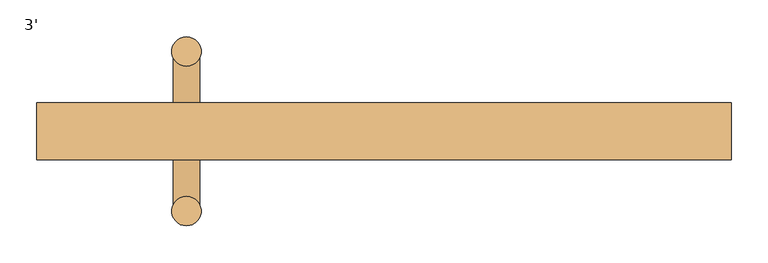
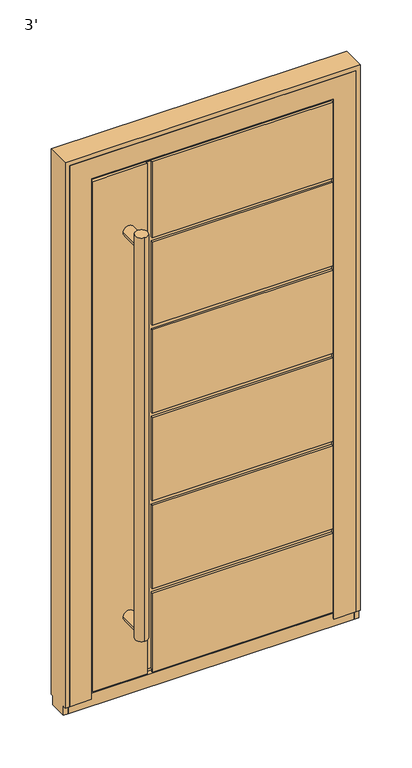
"""IFC4 building model written with IfcOpenShell, lengths in millimetres: door geometry, 3'."""

from ifc_helpers import new_model, si_unit, point, frame, frame_2d, origin, place, context, project, spatial, circle_curve, trimmed, segment, composite_curve, outline, extrude, faceted_brep, source, transform, mapped, element, save


def door_3_abbf6f65(model_context):
    return source(origin(), model_context, "Body", "SolidModel", [
        extrude(outline(composite_curve([segment(trimmed(circle_curve(frame_2d((-268.65, -52.7003001)), 20.0), [point((-268.65, -32.7003001))], [point((-268.65, -72.7003001))], False, "CARTESIAN"), True, "CONTINUOUS"), segment(trimmed(circle_curve(frame_2d((-268.65, -52.7003001)), 20.0), [point((-268.65, -72.7003001))], [point((-268.65, -32.7003001))], False, "CARTESIAN"), True, "CONTINUOUS")], self_intersect=False)), frame((0.0, 0.0, 210.0000003), z_axis=(0.0, 0.0, 1.0), x_axis=(1.0, 0.0, 0.0)), (0.0, 0.0, 1.0), 1363.8),
        extrude(outline(composite_curve([segment(trimmed(circle_curve(frame_2d((-268.65, 164.3003001)), 20.0), [point((-268.65, 184.3003001))], [point((-268.65, 144.3003001))], False, "CARTESIAN"), True, "CONTINUOUS"), segment(trimmed(circle_curve(frame_2d((-268.65, 164.3003001)), 20.0), [point((-268.65, 144.3003001))], [point((-268.65, 184.3003001))], False, "CARTESIAN"), True, "CONTINUOUS")], self_intersect=False)), frame((0.0, 0.0, 210.0000003), z_axis=(0.0, 0.0, 1.0), x_axis=(1.0, 0.0, 0.0)), (0.0, 0.0, 1.0), 1363.8),
        extrude(outline(composite_curve([segment(trimmed(circle_curve(frame_2d((241.9000003, -268.65)), 18.0), [point((241.9000003, -286.65))], [point((241.9000003, -250.65))], False, "CARTESIAN"), True, "CONTINUOUS"), segment(trimmed(circle_curve(frame_2d((241.9000003, -268.65)), 18.0), [point((241.9000003, -250.65))], [point((241.9000003, -286.65))], False, "CARTESIAN"), True, "CONTINUOUS")], self_intersect=False)), frame((0.0, -52.7, 0.0), z_axis=(0.0, 1.0, 0.0), x_axis=(0.0, 0.0, 1.0)), (0.0, 0.0, 1.0), 217.0),
        extrude(outline(composite_curve([segment(trimmed(circle_curve(frame_2d((1541.9000003, -268.65)), 18.0), [point((1541.9000003, -286.65))], [point((1541.9000003, -250.65))], False, "CARTESIAN"), True, "CONTINUOUS"), segment(trimmed(circle_curve(frame_2d((1541.9000003, -268.65)), 18.0), [point((1541.9000003, -250.65))], [point((1541.9000003, -286.65))], False, "CARTESIAN"), True, "CONTINUOUS")], self_intersect=False)), frame((0.0, -52.7, 0.0), z_axis=(0.0, 1.0, 0.0), x_axis=(0.0, 0.0, 1.0)), (0.0, 0.0, 1.0), 217.0),
        faceted_brep([(-193.65, 24.3, 306.466667), (-193.65, 24.3, 587.9333337), (383.65, 24.3, 587.9333337), (383.65, 24.3, 602.9333337), (-193.65, 24.3, 602.9333337), (-193.65, 24.3, 884.4000004), (383.65, 24.3, 884.4000004), (383.65, 24.3, 899.4000004), (-193.65, 24.3, 899.4000004), (-193.65, 24.3, 1180.866667), (383.65, 24.3, 1180.866667), (383.65, 24.3, 1195.866667), (-193.65, 24.3, 1195.866667), (-193.65, 24.3, 1477.3333337), (383.65, 24.3, 1477.3333337), (383.65, 24.3, 1492.3333337), (-193.65, 24.3, 1492.3333337), (-193.65, 24.3, 1748.8000003), (-208.65, 24.3, 1748.8000003), (-208.65, 24.3, 35.0), (-193.65, 24.3, 35.0), (-193.65, 24.3, 291.466667), (383.65, 24.3, 291.466667), (383.65, 24.3, 306.466667), (-193.65, 17.3, 306.466667), (-193.65, 17.3, 587.9333337), (383.65, 17.3, 587.9333337), (383.65, 26.3002302, 1748.8000003), (383.65, 17.3, 1748.8000003), (383.65, 17.3, 1492.3333337), (383.65, 17.3, 1477.3333337), (383.65, 17.3, 1195.866667), (383.65, 17.3, 1180.866667), (383.65, 17.3, 899.4000004), (383.65, 17.3, 884.4000004), (383.65, 17.3, 602.9333337), (383.65, 17.3, 306.466667), (383.65, 17.3, 291.466667), (383.65, 17.3, 24.0), (383.65, 19.2979528, 24.0), (383.65, 19.2979528, 35.0), (383.65, 26.3002302, 35.0), (-193.65, 17.3, 602.9333337), (-193.65, 17.3, 884.4000004), (-193.65, 17.3, 899.4000004), (-193.65, 17.3, 1180.866667), (-208.65, 17.3, 1748.8000003), (-208.65, 17.3, 24.0), (-208.65, 19.2979528, 24.0), (-208.65, 19.2979528, 35.0), (-193.65, 19.2979528, 35.0), (-383.65, 19.2979528, 35.0), (-383.65, 26.3002302, 35.0), (-193.65, 17.3, 291.466667), (-193.65, 19.2979528, 24.0), (-193.65, 17.3, 24.0), (-383.65, 19.2979528, 24.0), (-383.65, 17.3, 24.0), (-383.65, 17.3, 1748.8000003), (-193.65, 17.3, 1477.3333337), (-193.65, 17.3, 1195.866667), (-193.65, 17.3, 1748.8000003), (-193.65, 17.3, 1492.3333337), (408.65, 94.3, 10.0000003), (408.65, 91.3, 10.0000003), (-193.65, 91.3, 10.0000003), (-193.65, 94.3, 10.0000003), (-408.65, 91.3, 10.0000003), (-408.65, 94.3, 10.0000003), (-208.65, 94.3, 10.0000003), (-208.65, 91.3, 10.0000003), (408.65, 94.3, 291.466667), (408.65, 91.3, 291.466667), (408.65, 94.3, 306.466667), (408.65, 94.3, 587.9333337), (408.65, 91.3, 587.9333337), (408.65, 91.3, 306.466667), (408.65, 94.3, 899.4000004), (408.65, 94.3, 1180.866667), (408.65, 91.3, 1180.866667), (408.65, 91.3, 899.4000004), (408.65, 94.3, 602.9333337), (408.65, 94.3, 884.4000004), (408.65, 91.3, 884.4000004), (408.65, 91.3, 602.9333337), (408.65, 94.3, 1195.866667), (408.65, 94.3, 1477.3333337), (408.65, 91.3, 1477.3333337), (408.65, 91.3, 1195.866667), (408.65, 94.3, 1773.8000003), (408.65, 91.3, 1773.8000003), (408.65, 91.3, 1492.3333337), (408.65, 94.3, 1492.3333337), (393.15, 91.3, 291.466667), (393.15, 91.3, 25.5), (-193.65, 91.3, 25.5), (393.15, 91.3, 587.9333337), (393.15, 91.3, 306.466667), (393.15, 91.3, 1180.866667), (393.15, 91.3, 899.4000004), (393.15, 91.3, 884.4000004), (393.15, 91.3, 602.9333337), (393.15, 91.3, 1477.3333337), (393.15, 91.3, 1195.866667), (-193.65, 91.3, 1773.8000003), (-193.65, 91.3, 1758.3000003), (393.15, 91.3, 1758.3000003), (393.15, 91.3, 1492.3333337), (-393.15, 91.3, 25.5), (-393.15, 91.3, 1758.3000003), (-208.65, 91.3, 1758.3000003), (-208.65, 91.3, 1773.8000003), (-408.65, 91.3, 1773.8000003), (-208.65, 91.3, 25.5), (-193.65, 87.3, 291.466667), (-193.65, 94.3, 291.466667), (-193.65, 87.3, 25.5), (-193.65, 94.3, 306.466667), (-193.65, 94.3, 587.9333337), (-193.65, 94.3, 899.4000004), (-193.65, 94.3, 1180.866667), (-193.65, 94.3, 602.9333337), (-193.65, 94.3, 884.4000004), (-193.65, 94.3, 1195.866667), (-193.65, 94.3, 1477.3333337), (-193.65, 94.3, 1492.3333337), (-193.65, 94.3, 1773.8000003), (-408.65, 94.3, 1773.8000003), (-208.65, 94.3, 1773.8000003), (-208.65, 87.3, 1758.3000003), (-208.65, 87.3, 25.5), (-383.65, 26.3002302, 1748.8000003), (393.15, 26.3002302, 1758.3000003), (-393.15, 26.3002302, 1758.3000003), (-393.15, 26.3002302, 25.5), (393.15, 26.3002302, 25.5), (393.15, 87.3, 291.466667), (393.15, 87.3, 306.466667), (393.15, 87.3, 587.9333337), (393.15, 87.3, 602.9333337), (393.15, 87.3, 884.4000004), (393.15, 87.3, 899.4000004), (393.15, 87.3, 1180.866667), (393.15, 87.3, 1195.866667), (393.15, 87.3, 1477.3333337), (393.15, 87.3, 1492.3333337), (-193.65, 87.3, 1477.3333337), (-193.65, 87.3, 1195.866667), (-193.65, 87.3, 1180.866667), (-193.65, 87.3, 899.4000004), (-193.65, 87.3, 884.4000004), (-193.65, 87.3, 602.9333337), (-193.65, 87.3, 587.9333337), (-193.65, 87.3, 306.466667), (-193.65, 87.3, 1758.3000003), (-193.65, 87.3, 1492.3333337)], [[[0, 1, 2, 3, 4, 5, 6, 7, 8, 9, 10, 11, 12, 13, 14, 15, 16, 17, 18, 19, 20, 21, 22, 23]], [[1, 0, 24, 25]], [[1, 25, 26, 2]], [[27, 28, 29, 15, 14, 30, 31, 11, 10, 32, 33, 7, 6, 34, 35, 3, 2, 26, 36, 23, 22, 37, 38, 39, 40, 41]], [[42, 4, 3, 35]], [[5, 4, 42, 43]], [[5, 43, 34, 6]], [[44, 8, 7, 33]], [[9, 8, 44, 45]], [[19, 18, 46, 47, 48, 49]], [[41, 40, 50, 20, 19, 49, 51, 52]], [[53, 21, 20, 50, 54, 55]], [[21, 53, 37, 22]], [[24, 0, 23, 36]], [[40, 39, 54, 50]], [[56, 51, 49, 48]], [[39, 38, 55, 54]], [[57, 56, 48, 47]], [[33, 32, 45, 44]], [[35, 34, 43, 42]], [[36, 26, 25, 24]], [[55, 38, 37, 53]], [[58, 57, 47, 46]], [[31, 30, 59, 60]], [[28, 61, 62, 29]], [[63, 64, 65, 66]], [[67, 68, 69, 70]], [[64, 63, 71, 72]], [[73, 74, 75, 76]], [[77, 78, 79, 80]], [[81, 82, 83, 84]], [[85, 86, 87, 88]], [[89, 90, 91, 92]], [[65, 64, 72, 93, 94, 95]], [[76, 75, 96, 97]], [[80, 79, 98, 99]], [[84, 83, 100, 101]], [[88, 87, 102, 103]], [[90, 104, 105, 106, 107, 91]], [[108, 109, 110, 111, 112, 67, 70, 113]], [[114, 115, 66, 65, 95, 116]], [[63, 66, 115, 71]], [[74, 73, 117, 118]], [[78, 77, 119, 120]], [[82, 81, 121, 122]], [[86, 85, 123, 124]], [[89, 92, 125, 126]], [[68, 127, 128, 69]], [[68, 67, 112, 127]], [[129, 130, 113, 70, 69, 128, 111, 110]], [[58, 131, 52, 51, 56, 57]], [[132, 133, 134, 135], [131, 27, 41, 52]], [[106, 132, 135, 94, 93, 136, 137, 97, 96, 138, 139, 101, 100, 140, 141, 99, 98, 142, 143, 103, 102, 144, 145, 107]], [[94, 135, 134, 108, 113, 130, 116, 95]], [[133, 109, 108, 134]], [[146, 147, 143, 142, 148, 149, 141, 140, 150, 151, 139, 138, 152, 153, 137, 136, 114, 116, 130, 129, 154, 155, 145, 144]], [[149, 148, 120, 119]], [[149, 119, 77, 80, 99, 141]], [[122, 150, 140, 100, 83, 82]], [[151, 150, 122, 121]], [[151, 121, 81, 84, 101, 139]], [[118, 152, 138, 96, 75, 74]], [[153, 152, 118, 117]], [[153, 117, 73, 76, 97, 137]], [[115, 114, 136, 93, 72, 71]], [[9, 45, 32, 10]], [[60, 12, 11, 31]], [[13, 12, 60, 59]], [[13, 59, 30, 14]], [[62, 16, 15, 29]], [[16, 62, 61, 17]], [[124, 146, 144, 102, 87, 86]], [[125, 155, 154, 105, 104, 126]], [[120, 148, 142, 98, 79, 78]], [[147, 123, 85, 88, 103, 143]], [[147, 146, 124, 123]], [[155, 125, 92, 91, 107, 145]], [[90, 89, 126, 104]], [[127, 112, 111, 128]], [[132, 106, 105, 154, 129, 110, 109, 133]], [[27, 131, 58, 46, 18, 17, 61, 28]]]),
        faceted_brep([(-457.2, 94.3, 0.0), (-412.7, 94.3, 0.0), (-412.7, 85.3, 0.0), (-457.2, 85.2997571, 0.0), (-403.2, 21.8000042, 0.0), (-387.7, 21.8000042, 0.0), (-387.7, 17.3, 0.0), (-457.2, 17.3, 0.0), (-457.2, 26.3, 0.0), (-403.2, 26.3, 0.0), (457.2, 17.3, 0.0), (387.7, 17.3, 0.0), (387.7, 21.8000042, 0.0), (403.2, 21.8000042, 0.0), (403.2, 26.3, 0.0), (457.2, 26.3, 0.0), (412.7, 85.3, 0.0), (412.7, 94.3, 0.0), (457.2, 94.3, 0.0), (457.2, 85.2997571, 0.0), (-457.2, 17.3, 1828.8), (-457.2, 94.3, 1828.8), (-457.2, 85.2997571, -30.0), (-457.2, 26.3, -30.0), (457.2, 94.3, 1828.8), (412.7, 94.3, 1784.3), (-412.7, 94.3, 1784.3), (457.2, 17.3, 1828.8), (457.2, 26.3, -30.0), (457.2, 85.2997571, -30.0), (-387.7, 17.3, 1759.3), (387.7, 17.3, 1759.3), (-403.2, 85.3, 1774.8), (-403.2, 21.8000042, 1774.8), (-403.2, 26.3, 14.5), (-403.2, 85.3, 14.5), (403.2, 85.3, 1774.8), (403.2, 21.8000042, 1774.8), (403.2, 85.3, 14.5), (403.2, 26.3, 14.5), (-412.7, 85.3, 1784.3), (412.7, 85.3, 1784.3), (387.7, 21.8000042, 1759.3), (-387.7, 21.8000042, 1759.3)], [[[0, 1, 2, 3]], [[4, 5, 6, 7, 8, 9]], [[10, 11, 12, 13, 14, 15]], [[16, 17, 18, 19]], [[7, 20, 21, 0, 3, 22, 23, 8]], [[1, 0, 21, 24, 18, 17, 25, 26]], [[21, 20, 27, 24]], [[18, 24, 27, 10, 15, 28, 29, 19]], [[7, 6, 30, 31, 11, 10, 27, 20]], [[32, 33, 4, 9, 34, 35]], [[33, 32, 36, 37]], [[37, 36, 38, 39, 14, 13]], [[40, 2, 1, 26]], [[16, 19, 29, 22, 3, 2, 40, 41], [36, 32, 35, 38]], [[5, 4, 33, 37, 13, 12, 42, 43]], [[6, 5, 43, 30]], [[26, 25, 41, 40]], [[31, 30, 43, 42]], [[17, 16, 41, 25]], [[12, 11, 31, 42]], [[23, 28, 15, 14, 39, 34, 9, 8]], [[38, 35, 34, 39]], [[23, 22, 29, 28]]]),
        faceted_brep([(-457.2, 85.3, -30.0), (-457.2, 26.3, -30.0), (-472.2, 26.3, -30.0), (-472.2, 85.3, -30.0), (-457.2, 94.3, 1828.8), (-457.2, 17.3, 1828.8), (-457.2, 17.3, 0.0), (-457.2, 26.3, 0.0), (-457.2, 85.3, 0.0), (-457.2, 94.3, 0.0), (472.2, 26.3, 0.0), (457.2, 26.3, 0.0), (457.2, 26.3, -30.0), (472.2, 26.3, -30.0), (-472.2, 26.3, 0.0), (-472.2, 17.3, 1843.8), (-472.2, 94.3, 1843.8), (-472.2, 94.3, 0.0), (-472.2, 85.3, 0.0), (-472.2, 17.3, 0.0), (457.2, 85.3, 0.0), (472.2, 85.3, 0.0), (472.2, 85.3, -30.0), (457.2, 85.3, -30.0), (457.2, 17.3, 1828.8), (457.2, 94.3, 1828.8), (457.2, 94.3, 0.0), (457.2, 17.3, 0.0), (472.2, 94.3, 1843.8), (472.2, 94.3, 0.0), (472.2, 17.3, 0.0), (472.2, 17.3, 1843.8)], [[[0, 1, 2, 3]], [[4, 5, 6, 7, 1, 0, 8, 9]], [[10, 11, 12, 13]], [[7, 14, 2, 1]], [[15, 16, 17, 18, 3, 2, 14, 19]], [[20, 21, 22, 23]], [[18, 8, 0, 3]], [[24, 25, 26, 20, 23, 12, 11, 27]], [[25, 4, 9, 17, 16, 28, 29, 26]], [[21, 20, 26, 29]], [[8, 18, 17, 9]], [[22, 13, 12, 23]], [[11, 10, 30, 27]], [[14, 7, 6, 19]], [[5, 24, 27, 30, 31, 15, 19, 6]], [[28, 31, 30, 10, 13, 22, 21, 29]], [[5, 4, 25, 24]], [[16, 15, 31, 28]]]),
    ])


if __name__ == "__main__":
    model = new_model("IFC4")
    model_context = context("Model", 3, world=origin())
    ifc_project = project(units=[si_unit("LENGTHUNIT", "METRE", prefix="MILLI")], contexts=[model_context])
    site = spatial("IfcSite", under=ifc_project)
    building = spatial("IfcBuilding", under=site)
    placement = place(None, origin())
    door_3_shape = door_3_abbf6f65(model_context)
    element("IfcDoor", 1, ObjectType="3'", at=placement, inside=building, context=model_context, shape_type="MappedRepresentation", body=[
        mapped(door_3_shape, transform((0.0, 0.0, 0.0), x_axis=(1.0, 0.0, 0.0), y_axis=(0.0, 1.0, 0.0), z_axis=(0.0, 0.0, 1.0))),
    ])
    save(model, "model.ifc")

# Revit data of these elements
# Type "3'"
#   Type Mark = "9"
#   Water resistance = "up to Class E900, EN 12208:2001"
#   Uniclass2015Version = "v1.21"
#   Uniclass2015Reference = "Ss_25_30_20_30"
#   Uniclass2015Description = "Frame and door leaf system"
#   URL = "www.aluprof.com"
#   Type IFC Predefined Type = "USERDEFINED"
#   Right-hand / Left-hand door [instance default] = ""
#   Resistance to wind load = "up to Class C5/B5, EN 12210:2001"
#   Insert type = "ST"
#   Hardware [instance default] = ""
#   Product page = "https://aluprof.com/en/architects/offer/window-and-door-systems/panel-doors#visualisation"
#   Operation = "SinglePanelOutwardOpening"
#   Opening type = "Outward"
#   NBSReference = "25-50-20/125"
#   NBSDescription = "Frame and door leaf system"
#   Important = "The actual acceptable construction dimensions are dependent on the selection of profiles and hardware, glazing type, construction weight and the construction’s operating conditions. These should be determined by a suitably qualified person, and using ALUPROF’s calculation software"
#   IfcExportType = "USERDEFINED"
#   IfcExportAs = "IfcDoorType"
#   Handle type [instance default] = ""
#   Manufacturer = "ALUPROF SA"
#   Export Type to IFC As = "IfcDoorType"
#   Door sill type [instance default] = ""
#   Description = "External single-leaf panel door outward opening"
#   Model = "MB-86 ST Panel Door AD07"
#   Content of the recyclate in the material = "69.2%"
#   COBie.Type.WarrantyDurationParts = ""
#   COBie.Type.Name = ""
#   COBie.Type.Manufacturer = "ALUPROF SA"
#   COBie.Space.Name = ""
#   COBie.Floor.Name = ""
#   COBie.Facility.Name = ""
#   COBie.CreatedOn = ""
#   COBie.Component.WarrantyStartDate = ""
#   COBie.Component.Name = "MB-86 ST Panel Door AD07"
#   Burglar resistance = "RC2"
#   Air permeability = "up to Class 4, EN 12207:2001"
#   Width of the active leaf = 2' - 8.17717"
#   Placement in wall = 0' - 0.7874"
#   Thickness = 0' - 3.0315"
#   Height of the opening sash = 5' - 9.44094"
#   Handle Offset = 3' - 5.33858"
#   Rough Height = 6' - 2.40945"
#   Rough Width = 3' - 1.1811"
#   Height = 6' - 0"
#   Width = 3' - 0"
#   Construction depth = 0' - 3.0315"
#   Clear opening width = 2' - 3.94882"
#   Clear opening height = 5' - 8.47638"
#   Height of the array = 0' - 11.08136"
#   Schedule No. [instance default] = 1
#   Handrail [instance default] = yes
#   IsExternal = yes
#   Handle [instance default] = no
#   Door closer [instance default] = no
#   Function = 1
#   COBie.Type = yes
#   COBie = yes
#   Access control [instance default] = no
#   Panel = element 380416
#   Wall Closure = (empty or 0)
